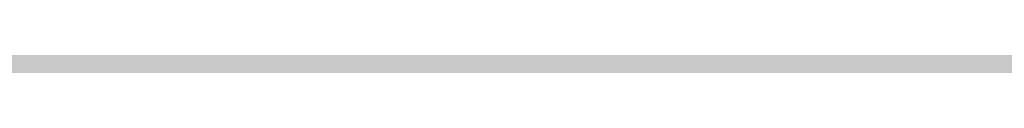
# Model space of a CAD drawing. Units: inches. Extents: x 2091 to 2899, y 967 to 2217.
# Tile 225 of 256: x 2203.4104 to 2203.7172, y 1152.2479 to 1152.2487. Entities that reach past the tile are written whole.
import ezdxf

# ---------------------------------------------------------------- set-up
doc = ezdxf.new("R2010")
doc.units = ezdxf.units.IN
doc.layers.add('A-WALL-PATT', color=141, linetype='Continuous', lineweight=13, true_color=0xadddf7)

msp = doc.modelspace()

# ---------------------------------------------------------------- hatches: boundary and pattern name
at = {"layer": 'A-WALL-PATT'}
h = msp.add_hatch(color=256, dxfattribs=at)
h.dxf.hatch_style = 1
h.paths.add_polyline_path([(2803.1436, 2050.91906), (2203.1436, 2050.91906), (2203.1436, 1090.91906), (2803.1436, 1090.91906)])
h.paths.add_polyline_path([(2635.79885, 1147.54046), (2674.52405, 1147.54046, 0.376086), (2678.52967, 1152.8802), (2678.52967, 1159.55647, 0.333335), (2674.52432, 1163.56185), (2674.52432, 1163.56185), (2674.52432, 1192.93439), (2635.80597, 1192.93439), (2597.08762, 1192.93439), (2597.08762, 1163.56185, 0.333335), (2593.08228, 1159.55647), (2593.08228, 1152.8802, 0.376086), (2597.08789, 1147.54046)], flags=0)
h.paths.add_polyline_path([(2436.01043, 1278.24078, 0.000483), (2435.95264, 1278.21503, -0.001328), (2435.93563, 1278.11169, -0.001711), (2436.11644, 1278.04076, 0.002185)], flags=0)
h.paths.add_polyline_path([(2794.1436, 1143.41906), (2794.1436, 1347.41906), (2543.37017, 1347.41906), (2543.37017, 1351.91906), (2794.1436, 1351.91906), (2794.1436, 1392.71355), (2793.9474, 1392.71355), (2793.9474, 1473.5369), (2794.1436, 1473.5369), (2794.1436, 1531.91906), (2650.1436, 1531.91906), (2650.1436, 1536.41906), (2794.1436, 1536.41906), (2794.1436, 1692.41906), (2609.37561, 1692.41906), (2609.37561, 1644.41906), (2604.87561, 1644.41906), (2604.87561, 1744.91906), (2609.37561, 1744.91906), (2609.37561, 1696.91906), (2794.1436, 1696.91906), (2794.1436, 1780.91906), (2609.6436, 1780.91906), (2493.87561, 1780.91906), (2493.87561, 1785.41906), (2609.6436, 1785.41906), (2794.1436, 1785.41906), (2794.1436, 1847.93882), (2793.95122, 1847.93882), (2793.95122, 1928.76217), (2794.1436, 1928.76217), (2794.1436, 1941.41906), (2614.1436, 1941.41906), (2614.1436, 1821.41906), (2609.6436, 1821.41906), (2609.6436, 1941.41906), (2392.1436, 1941.41906), (2392.1436, 1819.91906), (2387.6436, 1819.91906), (2387.6436, 1941.41906), (2212.1436, 1941.41906), (2212.1436, 1783.91906), (2392.1436, 1783.91906), (2392.1436, 1780.91906), (2212.1436, 1780.91906), (2212.1436, 1629.41906), (2387.6436, 1629.41906), (2387.6436, 1744.91906), (2392.1436, 1744.91906), (2392.1436, 1627.91906), (2317.1436, 1627.91906), (2317.1436, 1551.41906), (2317.1436, 1536.41906), (2459.38359, 1536.41906), (2459.38359, 1602.39648), (2463.88359, 1602.39648), (2463.88359, 1531.91906), (2456.6436, 1531.91906), (2456.6436, 1529.91906), (2452.1436, 1529.91906), (2452.1436, 1531.91906), (2312.6436, 1531.91906), (2312.6436, 1551.41906), (2306.1436, 1551.41906), (2306.1436, 1555.91906), (2308.1436, 1555.91906), (2308.1436, 1551.41906), (2312.6436, 1551.41906), (2312.6436, 1627.91906), (2212.1436, 1627.91906), (2212.1436, 1555.91906), (2270.1436, 1555.91906), (2270.1436, 1551.41906), (2212.1436, 1551.41906), (2212.1436, 1351.91906), (2272.1436, 1351.91906), (2272.1436, 1347.41906), (2212.1436, 1347.41906), (2212.1436, 1275.41906), (2308.1436, 1275.41906), (2308.1436, 1351.91906), (2452.1436, 1351.91906), (2452.1436, 1493.91906), (2456.6436, 1493.91906), (2456.6436, 1347.41906), (2312.6436, 1347.41906), (2312.6436, 1270.91906), (2212.1436, 1270.91906), (2212.1436, 1099.91906), (2281.23752, 1099.91906), (2282.87104, 1110.9138), (2282.00834, 1116.9966), (2278.55774, 1121.4204), (2268.20564, 1128.0562), (2272.08764, 1128.0562), (2273.81294, 1131.927), (2279.42034, 1134.6919), (2285.02784, 1135.2449), (2287.61584, 1137.4568), (2288.04714, 1138.0098), (2289.34114, 1140.7747), (2291.06654, 1139.6687), (2292.36054, 1135.2449), (2295.37984, 1136.9038), (2296.24254, 1135.7979), (2297.10524, 1133.033), (2300.12464, 1138.0098), (2303.14394, 1138.0098), (2304.43794, 1135.7979), (2303.14394, 1133.586), (2306.59464, 1134.6919), (2307.88874, 1133.033), (2310.90804, 1135.2449), (2313.92744, 1134.1389), (2315.62686, 1132.4271), (2308.32004, 1117.5496), (2290.20384, 1109.8079), (2288.90984, 1103.1721), (2289.27231, 1099.91906), (2434.91823, 1099.91906), (2431.59323, 1124.78806), (2429.93023, 1169.55306), (2430.92718, 1240.51969), (2435.65893, 1238.18613), (2437.13523, 1196.55406), (2438.79823, 1143.97306), (2442.67823, 1111.99806), (2446.55823, 1099.91906), (2794.1436, 1099.91906), (2794.1436, 1138.91906), (2548.03245, 1138.91906), (2548.03245, 1143.41906), (2548.03245, 1148.81906), (2546.66846, 1148.03156), (2528.68569, 1179.17862, 0.256256), (2512.03245, 1148.81906), (2512.03245, 1143.41906), (2512.03245, 1138.91906), (2507.53245, 1138.91906), (2507.53245, 1143.41906), (2507.53245, 1148.81906, 0.256256), (2490.8792, 1179.17862), (2472.89644, 1148.03156), (2471.53245, 1148.81906), (2471.53245, 1143.41906), (2467.03245, 1143.41906), (2467.03245, 1269.94579, 0.039061), (2460.90999, 1273.58006), (2467.03245, 1273.58006), (2467.03245, 1286.32536, 0.014511), (2465.21619, 1286.76191), (2467.03245, 1287.05258), (2467.03245, 1323.41906), (2471.53245, 1323.41906), (2471.53245, 1148.81906), (2489.53245, 1179.99597), (2490.89644, 1179.20847), (2490.8792, 1179.17862, -0.256256), (2507.53245, 1148.81906), (2507.53245, 1143.41906), (2512.03245, 1143.41906), (2512.03245, 1148.81906, -0.256256), (2528.68569, 1179.17862), (2528.66846, 1179.20847), (2530.03245, 1179.99597), (2548.03245, 1148.81906), (2548.03245, 1143.41906)], flags=16)
h.paths.add_polyline_path([(2607.76855, 1200.94508), (2607.76855, 1265.03063), (2597.08762, 1281.05201), (2619.78459, 1281.05201), (2627.79528, 1337.12686), (2635.79885, 1337.12686), (2643.81666, 1337.12686), (2651.82736, 1281.05201), (2674.52432, 1281.05201), (2663.8434, 1265.03063), (2663.8434, 1200.94508), (2635.80597, 1200.94508)], flags=0)
edge = h.paths.add_edge_path(flags=0)
edge.add_ellipse((13303.89622, 1272.99872), major_axis=(-10595.31304, 0), ratio=0.84230387009, start_angle=0.628237219, end_angle=0.6465541, ccw=False)
edge.add_ellipse((2711.70045, 1156.85268), major_axis=(2.21977, 0), ratio=0.8423039, start_angle=111.53524, end_angle=180.62824, ccw=False)
edge.add_ellipse((13303.15629, 1272.99872), major_axis=(-10593.02631, 0), ratio=0.84230386954, start_angle=0.528271472, end_angle=0.646554097, ccw=False)
edge.add_line((2710.7646, 1175.3333), (2710.12999, 1175.3333))
edge.add_ellipse((2710.12999, 1176.57978), major_axis=(1.47985, 0), ratio=0.8423039, start_angle=180, end_angle=270, ccw=False)
edge.add_line((2708.65014, 1176.57978), (2708.65014, 1200.78291))
edge.add_ellipse((2710.12999, 1200.78291), major_axis=(1.47985, 0), ratio=0.8423039, start_angle=90, end_angle=180, ccw=False)
edge.add_line((2710.12999, 1202.02939), (2710.46508, 1202.02939))
edge.add_ellipse((13303.15629, 1272.99872), major_axis=(-10593.02631, 0), ratio=0.84230386954, start_angle=-0.090229089, end_angle=0.383866779, ccw=False)
edge.add_ellipse((2710.12999, 1290.92703), major_axis=(-1.47985, 0), ratio=0.8423039, start_angle=0, end_angle=90, ccw=False)
edge.add_line((2708.65014, 1290.92703), (2708.65014, 1315.13017))
edge.add_ellipse((2710.12999, 1315.13017), major_axis=(-1.47985, 0), ratio=0.8423039, start_angle=-90, end_angle=0, ccw=False)
edge.add_line((2710.12999, 1316.37665), (2710.70631, 1316.37665))
edge.add_ellipse((3238.40172, 1296.28957), major_axis=(528.234, 0), ratio=0.84230387, start_angle=176.3495724, end_angle=177.8200497, ccw=False)
edge.add_ellipse((2775.06304, 1071.4507), major_axis=(313.30776, 0), ratio=0.84230387, start_angle=102.1259656, end_angle=103.780529, ccw=False)
edge.add_ellipse((2775.06304, 1078.3057), major_axis=(-305.30289, 0), ratio=0.84230387, start_angle=-79.790461, end_angle=-77.5553727, ccw=False)
edge.add_ellipse((2695.14177, 1541.97538), major_axis=(-250.96022, 0), ratio=0.84230387, start_angle=99.256566, end_angle=102.5549326)
edge.add_line((2741.41033, 1334.21426), (2747.13255, 1337.37848))
edge.add_ellipse((2747.53862, 1336.85748), major_axis=(-0.73992, 0), ratio=0.842304, start_angle=270, end_angle=307.93313, ccw=False)
edge.add_ellipse((2747.53862, 1336.85748), major_axis=(-0.73992, 0), ratio=0.842304, start_angle=232.06687, end_angle=270, ccw=False)
edge.add_line((2747.94469, 1337.37848), (2753.66691, 1334.21426))
edge.add_ellipse((2799.93547, 1541.97538), major_axis=(250.96022, 0), ratio=0.84230387, start_angle=257.4450674, end_angle=260.743434)
edge.add_ellipse((2720.01419, 1078.3057), major_axis=(305.30289, 0), ratio=0.84230387, start_angle=77.5553727, end_angle=79.790461, ccw=False)
edge.add_ellipse((2720.01419, 1071.4507), major_axis=(-313.30776, 0), ratio=0.84230387, start_angle=256.219471, end_angle=257.8740344, ccw=False)
edge.add_ellipse((2256.67551, 1296.28957), major_axis=(-528.234, 0), ratio=0.84230387, start_angle=182.1799503, end_angle=183.6504276, ccw=False)
edge.add_line((2784.37092, 1316.37665), (2784.94725, 1316.37665))
edge.add_ellipse((2784.94725, 1315.13017), major_axis=(1.47985, 0), ratio=0.8423039, start_angle=0, end_angle=90, ccw=False)
edge.add_line((2786.42709, 1315.13017), (2786.42709, 1290.92703))
edge.add_ellipse((2784.94725, 1290.92703), major_axis=(1.47985, 0), ratio=0.8423039, start_angle=270, end_angle=360, ccw=False)
edge.add_ellipse((-7808.07906, 1272.99872), major_axis=(10593.02631, 0), ratio=0.84230386954, start_angle=-0.383866779, end_angle=0.090229089, ccw=False)
edge.add_line((2784.61216, 1202.02939), (2784.94725, 1202.02939))
edge.add_ellipse((2784.94725, 1200.78291), major_axis=(1.47985, 0), ratio=0.8423039, start_angle=0, end_angle=90, ccw=False)
edge.add_line((2786.42709, 1200.78291), (2786.42709, 1176.57978))
edge.add_ellipse((2784.94725, 1176.57978), major_axis=(-1.47985, 0), ratio=0.8423039, start_angle=90, end_angle=180, ccw=False)
edge.add_line((2784.94725, 1175.3333), (2784.31264, 1175.3333))
edge.add_ellipse((-7808.07906, 1272.99872), major_axis=(10593.02631, 0), ratio=0.84230386954, start_angle=-0.618643196, end_angle=-0.528271472, ccw=False)
edge.add_ellipse((2783.37678, 1156.85268), major_axis=(-2.21977, 0), ratio=0.8423039, start_angle=179.37176, end_angle=248.46476, ccw=False)
edge.add_ellipse((-7808.81898, 1272.99872), major_axis=(-10595.31304, 0), ratio=0.84230386576, start_angle=179.353445923, end_angle=179.371762803, ccw=False)
edge.add_ellipse((2780.2973, 1153.50079), major_axis=(-5.24643, 0), ratio=0.8423039, start_angle=90, end_angle=179.35345, ccw=False)
edge.add_line((2780.2973, 1149.08171), (2714.77993, 1149.08171))
edge.add_ellipse((2714.77993, 1153.50079), major_axis=(5.24643, 0), ratio=0.8423039, start_angle=180.64655, end_angle=270, ccw=False)
edge = h.paths.add_edge_path(flags=0)
edge.add_line((2718.18737, 1151.00783), (2718.18737, 1170.47236))
edge.add_ellipse((2721.14706, 1170.47236), major_axis=(-2.95969, 0), ratio=0.8423039, start_angle=-90, end_angle=0, ccw=False)
edge.add_line((2721.14706, 1172.96532), (2773.93017, 1172.96532))
edge.add_ellipse((2773.93017, 1170.47236), major_axis=(-2.95969, 0), ratio=0.8423039, start_angle=180, end_angle=270, ccw=False)
edge.add_line((2776.88987, 1170.47236), (2776.88987, 1151.00783))
edge.add_line((2776.88987, 1151.00783), (2718.18737, 1151.00783))
edge = h.paths.add_edge_path(flags=0)
edge.add_line((2718.18737, 1180.23415), (2718.18737, 1199.05783))
edge.add_ellipse((2747.53862, 1320.39864), major_axis=(147.01792, 0), ratio=0.84230387, start_angle=256.4018653, end_angle=283.5981347)
edge.add_line((2776.88987, 1199.05783), (2776.88987, 1180.23415))
edge.add_ellipse((2747.53862, 1301.57496), major_axis=(147.01792, 0), ratio=0.84230387, start_angle=256.4018653, end_angle=283.5981347, ccw=False)
edge = h.paths.add_edge_path(flags=0)
edge.add_ellipse((13303.15629, 1272.99872), major_axis=(-10591.54646, 0), ratio=0.84230386955, start_angle=0.055594314, end_angle=0.377764194, ccw=False)
edge.add_line((2711.61686, 1262.72171), (2715.66741, 1249.4954))
edge.add_ellipse((6413.89196, 1241.69192), major_axis=(-3698.23616, 0), ratio=0.8423038695, start_angle=-0.12089737, end_angle=0.36407635)
edge.add_line((2715.76104, 1218.19245), (2711.93431, 1203.16736))
edge = h.paths.add_edge_path(flags=0)
edge.add_line((2718.18737, 1251.07457), (2716.00249, 1267.45044))
edge.add_ellipse((2742.15117, 1202.18954), major_axis=(81.77258, 0), ratio=0.84230387, start_angle=94.277421, end_angle=111.8349538, ccw=False)
edge.add_line((2737.00975, 1270.93063), (2758.06748, 1270.93063))
edge.add_ellipse((2752.92606, 1202.18954), major_axis=(81.77258, 0), ratio=0.84230387, start_angle=68.1650462, end_angle=85.722579, ccw=False)
edge.add_line((2779.07475, 1267.45044), (2776.88987, 1251.07457))
edge.add_ellipse((2750.33806, 1187.88536), major_axis=(79.57966, 0), ratio=0.84230387, start_angle=67.2080851, end_angle=85.1299304)
edge.add_line((2756.03466, 1254.74366), (2739.04258, 1254.74366))
edge.add_ellipse((2744.73917, 1187.88536), major_axis=(79.57966, 0), ratio=0.84230387, start_angle=94.8700696, end_angle=112.7919149)
edge = h.paths.add_edge_path(flags=0)
edge.add_line((2783.14293, 1203.16736), (2779.31619, 1218.19245))
edge.add_ellipse((-918.81473, 1241.69192), major_axis=(3698.23616, 0), ratio=0.8423038695, start_angle=-0.36407635, end_angle=0.12089737)
edge.add_line((2779.40983, 1249.4954), (2783.46037, 1262.72171))
edge.add_ellipse((-7808.07906, 1272.99872), major_axis=(-10591.54646, 0), ratio=0.84230386954, start_angle=179.622235806, end_angle=179.944405687, ccw=False)
edge = h.paths.add_edge_path(flags=0)
edge.add_ellipse((2734.20089, 1286.69044), major_axis=(-0.35661, 6.34008), ratio=0.6038336, start_angle=89.002014, end_angle=253.657408, ccw=False)
edge.add_line((2730.369, 1286.54181), (2730.369, 1301.35198))
edge.add_line((2730.369, 1301.35198), (2735.91331, 1305.2148))
edge.add_ellipse((2736.38492, 1304.73456), major_axis=(0.73992, 0), ratio=0.842304, start_angle=90, end_angle=134.48021, ccw=False)
edge.add_line((2736.38492, 1305.3578), (2738.03278, 1305.3578))
edge.add_line((2738.03278, 1305.3578), (2738.03278, 1307.70793))
edge.add_ellipse((2794.20164, 1307.70793), major_axis=(56.16886, 0), ratio=0.84230387, start_angle=150.56143, end_angle=180, ccw=False)
edge.add_ellipse((2700.87559, 1307.70793), major_axis=(-56.16886, 0), ratio=0.84230387, start_angle=180, end_angle=209.43857, ccw=False)
edge.add_line((2757.04445, 1307.70793), (2757.04445, 1305.3578))
edge.add_line((2757.04445, 1305.3578), (2758.69232, 1305.3578))
edge.add_ellipse((2758.69232, 1304.73456), major_axis=(-0.73992, 0), ratio=0.842304, start_angle=225.51979, end_angle=270, ccw=False)
edge.add_line((2759.16392, 1305.2148), (2764.70823, 1301.35198))
edge.add_line((2764.70823, 1301.35198), (2764.70823, 1286.54181))
edge.add_ellipse((2760.87634, 1286.69044), major_axis=(0.35661, 6.34008), ratio=0.6038336, start_angle=106.342592, end_angle=270.997986, ccw=False)
edge.add_line((2757.04445, 1285.79709), (2757.04445, 1307.70793))
edge.add_ellipse((2700.87559, 1307.70793), major_axis=(-56.16886, 0), ratio=0.84230387, start_angle=180, end_angle=209.43857)
edge.add_ellipse((2794.20164, 1307.70793), major_axis=(56.16886, 0), ratio=0.84230387, start_angle=150.56143, end_angle=180)
edge.add_line((2738.03278, 1307.70793), (2738.03278, 1285.79709))
h.paths.add_polyline_path([(2417.81227, 1104.4497), (2413.49227, 1102.5297), (2410.61227, 1103.9697), (2409.17227, 1106.3697), (2407.25227, 1107.3297), (2406.29227, 1109.7297), (2405.33227, 1114.0497), (2405.33227, 1117.8897), (2406.29227, 1120.1297), (2407.25227, 1119.8097), (2408.84832, 1118.32766), (2410.17395, 1119.42417), (2410.21127, 1120.4057), (2411.04073, 1121.41905), (2410.69927, 1119.8587), (2410.17395, 1119.42417), (2410.08845, 1117.17611), (2411.13284, 1116.20632), (2413.97227, 1119.3297), (2416.85227, 1120.7697), (2416.86972, 1120.79878), (2417.03507, 1119.40512), (2417.89621, 1118.14338), (2418.29227, 1118.3697), (2419.54445, 1120.03927), (2419.36092, 1118.38749), (2419.03211, 1119.35615), (2418.39894, 1118.51193), (2419.25227, 1114.5297), (2418.79409, 1107.19879)], flags=0)
h.paths.add_polyline_path([(2508.87017, 1347.41906), (2508.37017, 1347.41906), (2508.37017, 1351.91906), (2508.87017, 1351.91906)], flags=0)
h.paths.add_polyline_path([(2473.37017, 1347.41906), (2472.37017, 1347.41906), (2467.87017, 1347.41906), (2467.87017, 1455.41906), (2472.37017, 1455.41906), (2472.37017, 1352.41906), (2473.37017, 1352.41906)], flags=0)
h.paths.add_polyline_path([(2352.10624, 1217.4462), (2349.22624, 1218.8862), (2347.78624, 1221.2862), (2345.86624, 1222.2462), (2344.90624, 1224.6462), (2343.94624, 1228.9662), (2343.94624, 1232.8062), (2344.90624, 1235.0462), (2345.86624, 1234.7262), (2347.46229, 1233.24415), (2348.78792, 1234.34066), (2348.82524, 1235.3222), (2349.6547, 1236.33555), (2349.31324, 1234.7752), (2348.78792, 1234.34066), (2348.70242, 1232.0926), (2349.74681, 1231.12282), (2352.58624, 1234.2462), (2355.46624, 1235.6862), (2355.48369, 1235.71528), (2355.64904, 1234.32161), (2356.51018, 1233.05988), (2356.90624, 1233.2862), (2358.15842, 1234.95576), (2357.97489, 1233.30398), (2357.64608, 1234.27264), (2357.01291, 1233.42842), (2357.86624, 1229.4462), (2357.40806, 1222.11529), (2356.42624, 1219.3662)], flags=0)
h.paths.add_polyline_path([(2348.2968, 1112.22442), (2347.0138, 1112.31042), (2345.5298, 1114.12742), (2345.7318, 1115.85842), (2346.8118, 1116.98242), (2346.8118, 1114.64642), (2345.8668, 1114.21442), (2346.8798, 1114.30042)], flags=0)
h.paths.add_polyline_path([(2347.0138, 1110.92642), (2346.2718, 1110.49342), (2346.6098, 1111.18642)], flags=0)
h.paths.add_polyline_path([(2345.8668, 1118.19442), (2345.5298, 1117.32942), (2343.7078, 1118.02142), (2344.3828, 1118.62642)], flags=0)
h.paths.add_polyline_path([(2346.6768, 1109.28242), (2346.0698, 1108.07142), (2345.8668, 1110.06142)], flags=0)
h.paths.add_polyline_path([(2345.0568, 1119.75142), (2343.6398, 1119.75142), (2343.9778, 1121.13542)], flags=0)
h.paths.add_polyline_path([(2345.2598, 1116.55042), (2345.1248, 1115.85842), (2344.9218, 1115.68542), (2344.7198, 1116.37742)], flags=0)
h.paths.add_polyline_path([(2345.6648, 1112.31042), (2345.4618, 1111.53242), (2344.0448, 1111.96442), (2344.6518, 1112.57042)], flags=0)
h.paths.add_polyline_path([(2345.1918, 1113.34942), (2344.4498, 1113.86842), (2344.7198, 1114.38742)], flags=0)
h.paths.add_polyline_path([(2344.6518, 1116.80942), (2344.1798, 1115.68542), (2344.6518, 1115.33942), (2343.9098, 1114.90642), (2343.0328, 1115.94442), (2343.6398, 1116.46342)], flags=0)
h.paths.add_polyline_path([(2345.8668, 1106.68642), (2344.9898, 1105.56242), (2344.5168, 1106.60042)], flags=0)
h.paths.add_polyline_path([(2344.8548, 1110.06142), (2344.5168, 1109.28242), (2344.1128, 1109.71542)], flags=0)
h.paths.add_polyline_path([(2344.0448, 1113.52242), (2343.4378, 1113.08942), (2342.7628, 1113.95442)], flags=0)
h.paths.add_polyline_path([(2344.3148, 1111.01242), (2342.9648, 1110.32042), (2342.9648, 1111.09942)], flags=0)
h.paths.add_polyline_path([(2345.1248, 1104.69742), (2344.5848, 1103.74542), (2344.4498, 1104.26442)], flags=0)
h.paths.add_polyline_path([(2342.8298, 1121.22242), (2341.7498, 1120.53042), (2340.5358, 1121.04942), (2340.1308, 1121.82842), (2340.6708, 1122.95242), (2341.1428, 1121.82842), (2341.6148, 1122.00142)], flags=0)
h.paths.add_polyline_path([(2342.9648, 1119.75142), (2343.0328, 1118.45342), (2342.0878, 1118.02142), (2342.0198, 1119.49142)], flags=0)
h.paths.add_polyline_path([(2342.6948, 1116.89642), (2341.9528, 1116.63642), (2342.0198, 1117.32942)], flags=0)
h.paths.add_polyline_path([(2343.0328, 1112.22442), (2342.0198, 1111.79142), (2341.5478, 1112.22442), (2342.3578, 1113.34942)], flags=0)
h.paths.add_polyline_path([(2343.7748, 1104.43742), (2342.6278, 1102.88042), (2342.6948, 1104.61042), (2343.4378, 1105.12942)], flags=0)
h.paths.add_polyline_path([(2342.0198, 1115.07942), (2340.8058, 1115.51242), (2340.9408, 1116.37742)], flags=0)
h.paths.add_polyline_path([(2341.4808, 1120.09742), (2341.4808, 1119.40542), (2341.0758, 1119.57842), (2341.1428, 1120.09742)], flags=0)
h.paths.add_polyline_path([(2341.8178, 1114.47342), (2340.9408, 1113.08942), (2340.8058, 1114.56042)], flags=0)
h.paths.add_polyline_path([(2341.1428, 1118.54042), (2340.9408, 1116.98242), (2339.0508, 1117.67542), (2339.0508, 1118.62642)], flags=0)
h.paths.add_polyline_path([(2342.6948, 1101.66842), (2341.9528, 1101.84142), (2342.5598, 1102.36142)], flags=0)
h.paths.add_polyline_path([(2340.3328, 1119.66542), (2338.4438, 1119.57842), (2337.9038, 1120.35742), (2339.6578, 1120.61642)], flags=0)
h.paths.add_polyline_path([(2340.3328, 1115.33942), (2340.0628, 1113.69542), (2339.3878, 1115.33942)], flags=0)
h.paths.add_polyline_path([(2341.8178, 1103.83142), (2341.5478, 1102.88042), (2341.1428, 1103.65842)], flags=0)
h.paths.add_polyline_path([(2339.0508, 1122.86642), (2337.2958, 1121.82842), (2337.0938, 1123.12542), (2337.7688, 1123.81842)], flags=0)
h.paths.add_polyline_path([(2339.1178, 1121.74142), (2338.8478, 1121.22242), (2338.1738, 1121.04942), (2338.3758, 1121.56842)], flags=0)
h.paths.add_polyline_path([(2339.1858, 1119.31942), (2338.6458, 1118.71342), (2338.2408, 1118.10742), (2338.2408, 1118.88642)], flags=0)
h.paths.add_polyline_path([(2341.1428, 1101.92842), (2340.6028, 1101.23642), (2340.0628, 1101.84142), (2340.6028, 1102.36142)], flags=0)
h.paths.add_polyline_path([(2337.6338, 1117.76142), (2336.6208, 1118.28042), (2337.2958, 1118.97242)], flags=0)
h.paths.add_polyline_path([(2336.8238, 1119.57842), (2334.7988, 1118.97242), (2335.2038, 1120.35742), (2336.5538, 1120.87642)], flags=0)
h.paths.add_polyline_path([(2339.1178, 1100.45742), (2337.3638, 1100.54342), (2336.7558, 1101.23642)], flags=0)
h.paths.add_polyline_path([(2336.3508, 1122.43342), (2336.0138, 1121.91442), (2334.9338, 1122.43342), (2334.5288, 1123.47142), (2335.7438, 1122.77942)], flags=0)
h.paths.add_polyline_path([(2334.7318, 1120.87642), (2334.2588, 1120.35742), (2334.0568, 1120.78942), (2334.5968, 1121.30842)], flags=0)
h.paths.add_polyline_path([(2334.4618, 1122.17442), (2332.5718, 1121.30842), (2331.3568, 1122.17442), (2332.0998, 1122.86642)], flags=0)
h.paths.add_polyline_path([(2334.2588, 1118.54042), (2333.3818, 1118.45342), (2333.6518, 1119.31942)], flags=0)
h.paths.add_polyline_path([(2335.5418, 1102.27442), (2334.1918, 1102.62042), (2335.2718, 1103.31242)], flags=0)
h.paths.add_polyline_path([(2332.7068, 1119.66542), (2331.6948, 1120.44342), (2332.5048, 1120.78942)], flags=0)
h.paths.add_polyline_path([(2334.7318, 1101.14942), (2333.5168, 1101.58242), (2333.9888, 1101.75542)], flags=0)
h.paths.add_polyline_path([(2332.6398, 1116.63642), (2331.0868, 1116.29042), (2331.9648, 1118.19442)], flags=0)
h.paths.add_polyline_path([(2330.7498, 1121.56842), (2330.2768, 1120.27042), (2328.5228, 1119.31942), (2328.9948, 1121.04942)], flags=0)
h.paths.add_polyline_path([(2330.7498, 1118.62642), (2330.0078, 1117.50242), (2329.8728, 1118.02142)], flags=0)
h.paths.add_polyline_path([(2332.0998, 1102.36142), (2330.5468, 1102.01442), (2331.6948, 1102.96642)], flags=0)
h.paths.add_polyline_path([(2329.5348, 1113.60842), (2329.0628, 1112.31042), (2328.5898, 1113.34942)], flags=0)
h.paths.add_polyline_path([(2328.3878, 1117.84842), (2327.5098, 1116.55042), (2327.1728, 1117.76142)], flags=0)
h.paths.add_polyline_path([(2329.7378, 1106.51342), (2329.5348, 1105.30242), (2328.2528, 1106.08142)], flags=0)
h.paths.add_polyline_path([(2328.6578, 1114.38742), (2328.0498, 1114.12742), (2328.3198, 1114.90642)], flags=0)
h.paths.add_polyline_path([(2328.3198, 1112.22442), (2327.1058, 1112.13742), (2326.7008, 1112.65642)], flags=0)
h.paths.add_polyline_path([(2326.9028, 1115.25242), (2326.7008, 1114.12742), (2325.2158, 1113.60842), (2326.0928, 1115.33942)], flags=0)
h.paths.add_polyline_path([(2326.6328, 1108.33042), (2326.0928, 1107.37942), (2325.8908, 1108.50342), (2326.4978, 1109.10942)], flags=0)
h.paths.add_polyline_path([(2615.1436, 1531.91906), (2609.6436, 1531.91906), (2609.6436, 1620.41906), (2614.1436, 1620.41906), (2614.1436, 1536.41906), (2615.1436, 1536.41906)], flags=0)
h.paths.add_polyline_path([(2545.1436, 1563.41906), (2464.1436, 1563.41906), (2464.1436, 1632.41906), (2509.1436, 1632.41906), (2509.1436, 1627.91906), (2509.1436, 1603.91906), (2468.6436, 1603.91906), (2468.6436, 1567.91906), (2540.6436, 1567.91906), (2540.6436, 1591.91906), (2545.1436, 1591.91906)], flags=0)
h.paths.add_polyline_path([(2388.96905, 1549.98573), (2357.43418, 1549.98573), (2357.43418, 1623.36078), (2399.36278, 1623.36078), (2435.68947, 1623.36078), (2435.59255, 1602.55927), (2435.59255, 1602.39648), (2388.96905, 1602.39648)], flags=0)
h.paths.add_polyline_path([(2388.88063, 1555.80915), (2374.90443, 1555.80915), (2374.90443, 1600.57156), (2374.90443, 1615.45765), (2406.35088, 1615.45765), (2406.35088, 1618.93943), (2412.17429, 1615.45765), (2406.35088, 1611.97586), (2406.35088, 1615.45765), (2388.88063, 1615.45765)], flags=0)
h.paths.add_polyline_path([(2568.87561, 1644.41906), (2453.37561, 1644.41906), (2453.37561, 1785.41906), (2457.87561, 1785.41906), (2457.87561, 1648.91906), (2568.87561, 1648.91906)], flags=0)
h.paths.add_polyline_path([(2212.1436, 1945.91906), (2212.1436, 2041.91906), (2794.1436, 2041.91906), (2794.1436, 1945.91906)], flags=16)
h.paths.add_polyline_path([(2271.08273, 1964.31724), (2776.85297, 1964.31724), (2776.85297, 2037.16962), (2271.08273, 2037.16962)], flags=8)
h.paths.add_polyline_path([(2380.64929, 1536.82414), (2461.04081, 1536.82414), (2461.04081, 1554.65259), (2380.64929, 1554.65259)], flags=8)
h.paths.add_polyline_path([(2240.75571, 1609.72545), (2309.18583, 1609.72545), (2309.18583, 1617.6982), (2240.75571, 1617.6982)], flags=8)
h.paths.add_polyline_path([(2212.67726, 1313.5041), (2282.59152, 1313.5041), (2282.59152, 1322.74524), (2212.67726, 1322.74524)], flags=8)
h.paths.add_polyline_path([(2457.11198, 1114.77857), (2558.48158, 1114.77857), (2558.48158, 1142.21968), (2457.11198, 1142.21968)], flags=8)
h.paths.add_polyline_path([(2473.44234, 1273.01007), (2604.64123, 1273.01007), (2604.64123, 1318.34693), (2473.44234, 1318.34693)], flags=8)
h.paths.add_polyline_path([(2638.8763, 1626.97743), (2684.25037, 1627.97674), (2684.03848, 1637.59749), (2638.66442, 1636.59819)], flags=8)
h.paths.add_polyline_path([(2537.59055, 1453.79345), (2628.38955, 1453.79345), (2628.38955, 1475.34481), (2537.59055, 1475.34481)], flags=8)
h.paths.add_polyline_path([(2504.13764, 1714.6324), (2554.64719, 1714.6324), (2554.64719, 1730.23771), (2504.13764, 1730.23771)], flags=8)
h.paths.add_polyline_path([(2487.50118, 1575.65187), (2535.09712, 1575.65187), (2535.09712, 1598.37765), (2487.50118, 1598.37765)], flags=8)
h.paths.add_polyline_path([(2709.0994, 1735.71028), (2740.0166, 1735.71028), (2740.0166, 1749.93764), (2709.0994, 1749.93764)], flags=8)
h.paths.add_polyline_path([(2442.43842, 1792.17166), (2564.72884, 1792.17166), (2564.72884, 1842.00016), (2442.43842, 1842.00016)], flags=8)
h.paths.add_polyline_path([(2655.8158, 1809.64408), (2789.52014, 1806.6938), (2790.08498, 1832.29164), (2656.38064, 1835.24192)], flags=8)
h.paths.add_polyline_path([(2234.8427, 1797.72014), (2368.59285, 1794.76885), (2369.16072, 1820.50413), (2235.41056, 1823.45542)], flags=8)
h.paths.add_polyline_path([(2245.13847, 1644.00633), (2398.42773, 1640.6239), (2398.99484, 1666.32482), (2245.70557, 1669.70725)], flags=8)
h.paths.add_polyline_path([(2306.14285, 1431.16852), (2413.76831, 1428.79369), (2414.33315, 1454.39153), (2306.70768, 1456.76636)], flags=8)
h.paths.add_polyline_path([(2306.83458, 1458.23314), (2393.38048, 1456.32345), (2393.93281, 1481.35436), (2307.38691, 1483.26405)], flags=8)

doc.saveas('drawing.dxf')
